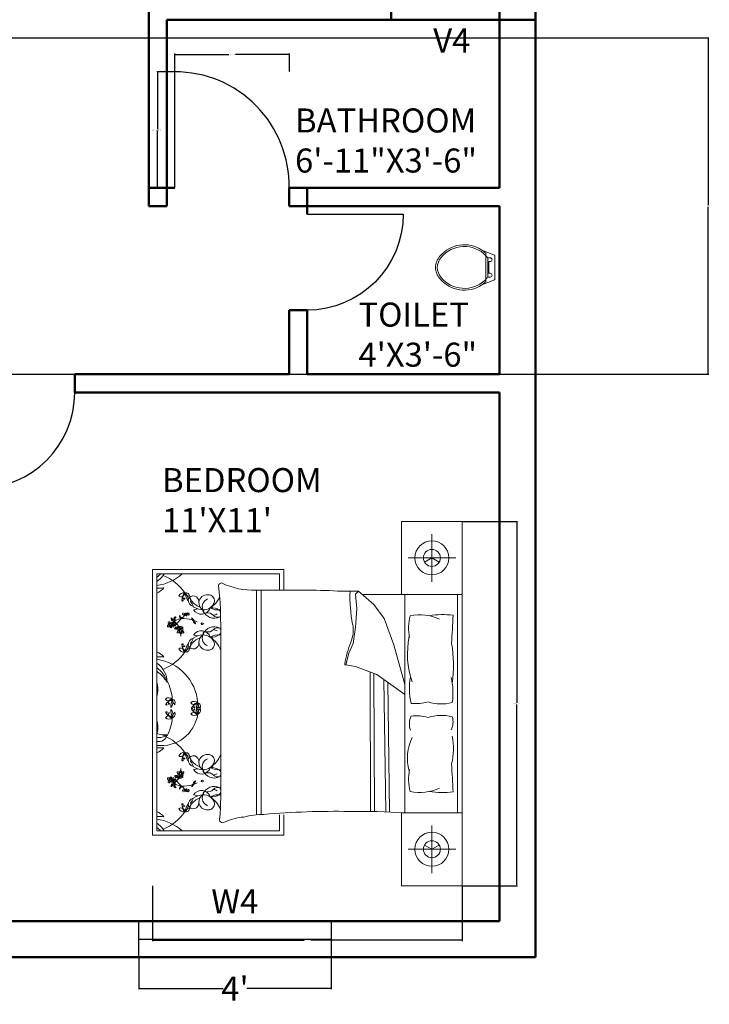
# Model space of a CAD drawing. Units: inches. Extents: x -173 to 545, y -746 to 104.
# Tile 19 of 32: x 373 to 545, y -709 to -463. Entities that reach past the tile are written whole.
import ezdxf

# ---------------------------------------------------------------- set-up
doc = ezdxf.new("R2010")
doc.units = ezdxf.units.IN
doc.header["$MEASUREMENT"] = 0
for name, color, linetype, lineweight in [('A-ANNO-DIMS', 2, 'Continuous', 18), ('A-ANNO-TEXT', 7, 'Continuous', 18), ('A-AREA-IDEN', 7, 'Continuous', 18), ('A-DOOR', 4, 'Continuous', 25), ('A-FLOR-FIXT', 8, 'Continuous', 18), ('A-FURN', 8, 'Continuous', 18), ('A-GLAZ', 3, 'Continuous', 25), ('A-WALL', 7, 'Continuous', 50)]:
    doc.layers.add(name, color=color, linetype=linetype, lineweight=lineweight)
doc.styles.get("Standard").update_dxf_attribs({"font": 'arial.ttf'})
doc.dimstyles.get("Standard").update_dxf_attribs({"dimtxt": 0.18, "dimasz": 0.18, "dimexe": 0.18, "dimexo": 0.0625, "dimgap": 0.09, "dimtad": 0, "dimtih": 1, "dimtoh": 1, "dimdec": 0, "dimzin": 0, "dimdsep": 46, "dimlunit": 3, "dimtxsty": 'Standard', "dimcen": 0.09, "dimadec": 0, "dimazin": 0, "dimtfac": 1, "dimtdec": 0, "dimtofl": 0, "dimtmove": 0, "dimatfit": 3, "dimfxl": 1, "dimtolj": 1, "dimtzin": 0, "dimarcsym": 0})

# ---------------------------------------------------------------- blocks, each defined once
blk = doc.blocks.new('*D20')
at = {"layer": 'A-ANNO-DIMS', "color": 0, "lineweight": -2, "transparency": 16777216}
for p, q in [((402.8, -697.42), (402.8, -705.33)), ((450.8, -697.42), (450.8, -705.33)), ((402.98, -705.15), (423.83, -705.15)), ((450.62, -705.15), (429.77, -705.15))]:
    blk.add_line(p, q, dxfattribs=at)
at = {"layer": 'A-ANNO-DIMS', "color": 0, "transparency": 16777216}
for points in [[(402.98, -705.12), (402.98, -705.18), (402.8, -705.15)], [(450.62, -705.12), (450.62, -705.18), (450.8, -705.15)]]:
    blk.add_solid(points, dxfattribs=at)
at = {"layer": 'Defpoints', "color": 0, "transparency": 16777216}
for p in [(402.8, -697.36), (450.8, -697.36), (450.8, -705.15)]:
    blk.add_point(p, dxfattribs=at)
at = {"layer": 'A-ANNO-DIMS', "color": 0, "transparency": 16777216, "insert": (426.8, -705.15), "char_height": 6, "attachment_point": 5}
blk.add_mtext("\\A1;4'", dxfattribs=at)
blk = doc.blocks.new('BED-SUITE-LARGE')
for p, q in [((77.28, 90.87), (77.28, 0)), ((69.71, 75.85), (69.71, 87.72)), ((63.77, 81.79), (75.65, 81.79)), ((0, 78.88), (32.74, 78.88)), ((0, 12.63), (0, 78.88)), ((32.74, 78.88), (32.74, 73.74)), ((1.05, 77.83), (1.05, 13.68)), ((31.68, 77.83), (1.05, 77.83)), ((31.68, 73.74), (31.68, 77.83)), ((25.93, 17.68), (25.93, 73.75)), ((27.07, 17.76), (27.07, 73.75)), ((50.66, 72.78), (51.39, 73.51)), ((51.02, 69.09), (50.66, 72.78)), ((51.39, 73.51), (55.25, 70.2)), ((77.28, 72.7), (52.34, 72.7)), ((62.92, 72.7), (62.92, 18.17)), ((76.12, 18.17), (76.12, 72.7)), ((10.27, 68.87), (11.29, 69.07)), ((50.66, 64.49), (51.02, 69.09)), ((55.25, 70.2), (57.83, 66.7)), ((57.83, 66.7), (60.22, 60.08)), ((50.1, 60.44), (50.66, 64.49)), ((10.27, 62.52), (11.29, 62.32)), ((17.01, 26.99), (17.01, 63.88)), ((49, 58.05), (50.1, 60.44)), ((60.22, 60.08), (62.92, 50.17)), ((48.26, 55.11), (49, 58.05)), ((50.66, 54.74), (48.26, 55.11)), ((55.99, 52.71), (50.66, 54.74)), ((54.42, 18.5), (54.28, 53.36)), ((55.35, 18.5), (55.22, 53.01)), ((62.92, 47.73), (55.99, 52.71)), ((58.21, 18.45), (57.75, 51.45)), ((59.15, 18.42), (58.69, 50.77)), ((10.27, 28.99), (11.29, 29.19)), ((10.27, 22.64), (11.29, 22.44)), ((31.68, 13.68), (31.68, 17.69)), ((32.74, 17.67), (32.74, 12.63)), ((69.71, 15.02), (69.71, 3.15)), ((32.74, 12.63), (0, 12.63)), ((1.05, 13.68), (31.68, 13.68)), ((63.77, 9.09), (75.65, 9.09))]:
    blk.add_line(p, q)
for points in [[(62.14, 72.7), (62.14, 90.87), (77.28, 90.87)], [(69.71, 81.79), (67.87, 80.73)], [(69.71, 81.79), (71.55, 80.73)], [(77.28, 18.17), (62.14, 18.17), (62.14, 0), (77.28, 0)], [(69.71, 9.09), (67.87, 10.15)], [(69.71, 9.09), (71.55, 10.15)]]:
    blk.add_lwpolyline(points)
for points in [[(43.07, 73.7, 0.001242), (25.83, 73.75, -0.127202), (17.23, 75.57)], [(75.02, 67.48, 0.074897), (69.08, 67.37, -0.472817)], [(68.75, 45.86, 0.14099), (74.8, 45.68, 0.235245)], [(68.75, 41.98, -0.14099), (74.8, 42.16, -0.235245)], [(75.02, 23.39, -0.074897), (69.08, 23.5, 0.472817)], [(27.78, 17.79, 0.056112), (22.78, 17.13, 0.095341), (17.97, 15.85)]]:
    blk.add_lwpolyline(points, format="xyb")
for centre, radius in [((69.71, 81.79), 4.24), ((69.71, 81.79), 2.12), ((4.53, 65.13), 0.231), ((6.97, 63.62), 0.231), ((6.97, 27.89), 0.231), ((4.53, 26.37), 0.231), ((69.71, 9.09), 4.24), ((69.71, 9.09), 2.12)]:
    blk.add_circle(centre, radius)
for centre, radius, start, end in [((-3.21, 82.79), 7.21, 306.3036, 316.4814), ((-2.13, 80.71), 5.78, 303.4617, 330.1116), ((-0.55, 86.66), 11.87, 277.745, 311.8856), ((-1.72, 66.36), 11.87, 34.3865, 68.5908), ((-0.8, 77.47), 4.82, 292.5547, 318.9546), ((1.8, 90.69), 16.42, 267.4081, 273.6519), ((17.29, 74.73), 0.838, 93.98, 207.3412), ((-77.59, 64.97), 94.6, 359.3433, 5.6887), ((7.79, 71.77), 1.32, 77.7115, 159.0387), ((7.08, 73.09), 0.991, 238.4633, 358.2869), ((10.33, 71.08), 3, 138.8402, 177.9352), ((7.56, 71.2), 0.0716, 11.4834, 127.9409), ((8.52, 72.2), 0.971, 117.6827, 223.7762), ((7.92, 71.62), 0.128, 223.7762, 159.7183), ((8.31, 72.1), 0.984, 2.9516, 103.728), ((16.18, 74.86), 8.3, 192.5173, 207.1824), ((6.98, 71.54), 1.88, 345.4653, 54.2343), ((9.8, 74.12), 2.03, 211.3827, 255.2969), ((10.19, 70.95), 1.36, 350.264, 160.8688), ((10.6, 71.28), 1.7, 175.969, 254.3045), ((8.71, 71.23), 0.836, 333.9755, 53.2681), ((13.19, 73.65), 4.29, 211.2614, 251.7045), ((13.69, 70.45), 2.17, 84.9449, 172.8857), ((14.51, 69.6), 2.11, 111.5819, 201.4221), ((13.91, 71.08), 1.53, 354.4856, 91.0538), ((10.61, 75.09), 6.88, 303.6671, 333.2997), ((49.13, 156.83), 83.35, 265.8294, 271.553), ((83.57, 71.96), 34.3, 177.4519, 191.3392), ((7.48, 71.19), 0.147, 177.9352, 11.4834), ((8.34, 69.44), 1.81, 6.1662, 51.5825), ((12.85, 73.69), 4.88, 236.2883, 266.5076), ((12.22, 70), 2.26, 209.9085, 343.1337), ((14.17, 70.83), 2.64, 182.3591, 234.0401), ((12.78, 71.55), 2.73, 265.2933, 346.921), ((14.7, 65.87), 3.5, 122.7011, 126.3445), ((16.34, 72.56), 3.76, 238.8218, 279.1554), ((14.7, 65.87), 3.5, 55.785, 94.7304), ((4.87, 66.63), 0.258, 124.3538, 214.3923), ((5.25, 66.59), 0.602, 190.3057, 287.1958), ((5.42, 66.8), 0.7, 176.9701, 248.2913), ((10.42, 70.49), 6.76, 212.6784, 216.3746), ((5.19, 66.64), 0.268, 216.3746, 291.7548), ((5.83, 66.45), 0.602, 122.8155, 187.3992), ((5.36, 66.2), 0.202, 289.3605, 111.7548), ((6.09, 66.37), 0.7, 109.4799, 177.6828), ((5.72, 66.82), 0.258, 56.8636, 146.9021), ((5.85, 66.53), 0.268, 148.8844, 224.2646), ((11.41, 63.17), 6.76, 145.1882, 148.8844), ((7.56, 62.88), 3.77, 94.756, 119.2041), ((15.59, 57.45), 12.42, 132.2412, 142.1744), ((9.32, 67.33), 2.56, 178.3264, 187.1302), ((6.55, 66.98), 0.477, 11.3256, 64.4621), ((8.17, 67.67), 1.44, 190.2588, 210.656), ((7.21, 67.08), 0.436, 188.3432, 274.2869), ((7.59, 67.32), 0.762, 210.656, 242.6341), ((8.17, 67.98), 1.46, 218.2101, 226.3071), ((7.09, 66.75), 0.185, 325.7657, 67.4417), ((1.34, 72.94), 8.63, 313.1541, 322.0459), ((7.74, 59.14), 7.53, 73.5842, 93.8277), ((7.69, 67.76), 0.178, 142.4737, 265.053), ((7.92, 67.79), 0.382, 127.7621, 169.0403), ((7.72, 68.11), 0.538, 265.053, 338.3618), ((8.43, 67.38), 0.703, 113.4276, 137.6104), ((8.35, 68.11), 0.231, 183.2768, 356.7232), ((8.52, 67.69), 0.379, 139.7889, 227.6792), ((8.4, 67.56), 0.199, 227.6792, 350.3487), ((7.63, 67.69), 0.758, 353.0852, 15.7171), ((8.12, 67.6), 0.478, 350.3487, 43.6538), ((9.01, 68.1), 0.557, 198.7263, 262.5032), ((8.57, 67.84), 0.221, 1.1081, 91.8675), ((8.71, 67.79), 0.386, 11.5637, 52.6358), ((8.98, 67.72), 0.179, 255.2356, 54.9248), ((12.38, 66.79), 2.56, 178.3264, 187.1302), ((9.61, 66.44), 0.477, 11.3256, 64.4621), ((11.23, 67.12), 1.44, 190.2588, 210.656), ((10.27, 66.54), 0.436, 188.3432, 274.2869), ((10.65, 66.78), 0.762, 210.656, 242.6341), ((11.23, 67.43), 1.46, 218.2101, 226.3071), ((10.15, 66.21), 0.185, 325.7657, 67.4417), ((13.17, 68.57), 0.564, 167.3041, 285.1471), ((15.36, 69.65), 2.9, 199.2822, 299.1751), ((13.81, 66.22), 1.86, 41.5653, 105.1471), ((14.83, 70.08), 2.61, 277.436, 299.9149), ((16.22, 68.36), 1.36, 221.5653, 293.8354), ((16, 67.9), 1.09, 30.0293, 52.325), ((16, 67.9), 1.09, 314.4517, 333.558), ((76.08, 64.24), 12.18, 165.1039, 191.0369), ((66.7, 55.9), 11.71, 65.1316, 101.7583), ((939.83, 17.39), 866.26, 176.68521, 177.14978), ((3.87, 64.78), 0.178, 142.4737, 265.053), ((4.11, 64.82), 0.382, 61.2196, 169.0403), ((3.9, 65.14), 0.538, 265.053, 338.3618), ((4.36, 65.61), 0.457, 157.4086, 261.4386), ((4.1, 65.62), 0.229, 58.0499, 135.6268), ((4.61, 64.41), 0.703, 113.4276, 137.6104), ((4.34, 65.48), 0.153, 172.906, 277.132), ((3.83, 65.2), 0.73, 14.7558, 58.0499), ((4.7, 64.72), 0.379, 139.7889, 227.6792), ((4.58, 64.58), 0.199, 227.6792, 350.3487), ((4.86, 65.39), 0.316, 36.1046, 181.4281), ((3.81, 64.72), 0.758, 353.0852, 15.7171), ((4.31, 64.63), 0.478, 350.3487, 43.6538), ((4.67, 65.64), 0.319, 270.0645, 331.1507), ((4.94, 65.56), 0.364, 221.8413, 265.7877), ((5.19, 65.12), 0.557, 198.7263, 262.5032), ((4.75, 64.86), 0.221, 1.1081, 91.8675), ((4.94, 65.42), 0.227, 263.7526, 41.7054), ((4.89, 64.81), 0.386, 11.5637, 86.365), ((7.56, 62.88), 3.77, 124.0033, 132.4917), ((5.17, 64.75), 0.179, 255.2356, 54.9248), ((3.67, 62.41), 4.03, 63.7819, 68.2913), ((5.83, 65.51), 0.641, 128.3208, 208.8162), ((5.94, 65.56), 0.766, 207.7043, 254.3516), ((5.51, 66.2), 0.202, 221.8703, 44.2646), ((6.43, 65.62), 1.05, 157.2305, 229.0635), ((6.07, 65.96), 0.621, 174.4544, 220.6188), ((5.44, 65.12), 1.05, 270.278, 342.111), ((6.15, 63.8), 0.746, 98.7227, 159.3375), ((5.77, 64.76), 0.766, 244.9899, 291.6373), ((2.54, 62.5), 4.53, 30.544, 49.818), ((5.04, 65.07), 0.746, 340.0041, 40.6188), ((5.94, 65.15), 0.621, 278.7227, 324.8872), ((5.83, 64.65), 0.641, 290.5253, 358.5375), ((6.8, 64.09), 0.457, 157.4086, 261.4386), ((6.54, 64.11), 0.229, 58.0499, 135.6268), ((7.08, 64.83), 0.641, 182.8499, 266.1226), ((6.83, 65.28), 0.621, 231.7607, 277.9252), ((7.32, 65.39), 1.05, 214.5369, 286.3699), ((6.78, 63.96), 0.153, 172.906, 277.132), ((6.27, 63.68), 0.73, 14.7558, 58.0499), ((2.54, 62.5), 4.53, 23.0501, 23.8477), ((7.02, 63.93), 0.746, 37.3105, 97.9252), ((7.3, 63.88), 0.316, 36.1046, 181.4281), ((7.11, 64.95), 0.766, 265.0106, 311.658), ((7.11, 64.12), 0.319, 270.0645, 331.1507), ((7.38, 63.91), 0.227, 263.7526, 41.7054), ((10.67, 65.87), 0.436, 147.5332, 233.4768), ((11.06, 66.09), 0.762, 179.1859, 211.164), ((10.32, 65.92), 0.185, 354.3784, 96.0543), ((7.74, 59.14), 7.53, 63.0032, 69.8941), ((11.64, 66.44), 1.44, 211.164, 231.5612), ((11.89, 67.61), 2.56, 234.6898, 243.4936), ((11.91, 66.29), 1.46, 195.5129, 203.6099), ((10.27, 65.34), 0.477, 357.3579, 50.4944), ((12.32, 65.43), 0.175, 12.7051, 190.4384), ((12.43, 65.45), 0.285, 190.4384, 10.4136), ((15.36, 61.74), 2.9, 60.8249, 160.7178), ((13.81, 65.17), 1.86, 254.8529, 318.4347), ((14.83, 61.31), 2.61, 60.0851, 82.564), ((16.22, 63.03), 1.36, 66.1646, 138.4347), ((16, 63.49), 1.09, 23.229, 45.5483), ((42.69, 63.76), 7.4, 336.2616, 11.3392), ((6.31, 63.27), 0.178, 142.4737, 265.053), ((6.54, 63.31), 0.382, 61.2196, 169.0403), ((6.34, 63.63), 0.538, 265.053, 338.3618), ((7.05, 62.89), 0.703, 113.4276, 137.6104), ((7.14, 63.2), 0.379, 139.7889, 227.6792), ((7.02, 63.07), 0.199, 227.6792, 350.3487), ((6.25, 63.21), 0.758, 353.0852, 15.7171), ((2.54, 62.5), 4.53, 357.1071, 4.7585), ((6.75, 63.12), 0.478, 350.3487, 43.6538), ((7.38, 64.05), 0.364, 221.8413, 265.7877), ((7.63, 63.61), 0.557, 198.7263, 262.5032), ((7.19, 63.35), 0.221, 1.1081, 91.8675), ((7.33, 63.3), 0.386, 11.5637, 86.365), ((7.61, 63.23), 0.179, 255.2356, 54.9248), ((10.6, 60.11), 1.7, 105.6955, 184.031), ((8.34, 61.95), 1.81, 308.4175, 353.8338), ((13.19, 57.74), 4.29, 108.2955, 148.7386), ((12.85, 57.7), 4.88, 93.4924, 123.7117), ((12.22, 61.39), 2.26, 16.8663, 150.0915), ((14.17, 60.56), 2.64, 125.9599, 177.6409), ((14.51, 61.79), 2.11, 158.5779, 248.4181), ((12.78, 59.84), 2.73, 13.079, 94.7067), ((13.17, 62.82), 0.564, 74.8529, 192.6959), ((14.7, 65.52), 3.5, 233.6555, 237.2989), ((16.34, 58.83), 3.76, 79.7133, 121.1782), ((14.7, 65.52), 3.5, 265.2696, 304.215), ((10.61, 56.3), 6.88, 21.4941, 56.3329), ((16, 63.49), 1.09, 307.675, 336.7144), ((84.74, 57.83), 21.12, 168.0397, 199.2615), ((7.08, 58.3), 0.991, 1.7131, 121.5367), ((7.79, 59.62), 1.32, 200.9613, 282.2885), ((7.48, 60.2), 0.147, 348.5166, 182.0648), ((10.33, 60.31), 3, 182.0648, 221.1598), ((7.56, 60.19), 0.0716, 232.0591, 348.5166), ((8.52, 59.19), 0.971, 136.2238, 242.3173), ((7.97, 59.76), 0.0774, 200.2667, 136.2271), ((6.98, 59.85), 1.88, 305.7657, 14.5347), ((16.18, 56.53), 8.3, 152.8176, 167.4827), ((8.31, 59.29), 0.984, 256.272, 357.0484), ((9.8, 57.27), 2.03, 104.7031, 148.6173), ((10.19, 60.44), 1.36, 199.1312, 9.736), ((8.71, 60.16), 0.836, 306.7319, 26.0245), ((13.69, 60.94), 2.17, 187.1143, 275.0551), ((13.91, 60.31), 1.53, 268.9462, 5.5144), ((82.6, 48.8), 35.24, 160.1194, 169.3383), ((42.13, 55.03), 32.96, 352.2196, 9.497), ((-0.8, 53.92), 4.82, 41.0454, 67.4453), ((1.8, 40.7), 16.42, 86.3481, 92.5919), ((-1.72, 65.03), 11.87, 291.4092, 325.6135), ((-0.55, 44.73), 11.87, 4.4623, 82.255), ((-2.13, 50.68), 5.78, 1.272, 56.5383), ((-3.21, 48.6), 7.21, 17.8504, 53.6964), ((48.19, 55.31), 0.219, 178.8623, 289.7536), ((-5.24, 44.82), 10.72, 34.0123, 54.053), ((80.12, 49.28), 16.03, 169.8617, 193.6238), ((58.79, 48.07), 16.19, 351.5249, 13.96), ((-5.19, 48.96), 6.53, 343.5431, 17.0202), ((-6.9, 45.64), 11.87, 4.4623, 27.4146), ((-8.55, 46.37), 9.65, 4.3787, 5.6357), ((-15.16, 41.29), 17.24, 19.7217, 19.9028), ((4.04, 45.59), 1.32, 47.7873, 129.1145), ((4.09, 47.08), 0.991, 208.5391, 328.3627), ((3.48, 45.23), 0.147, 148.011, 341.5592), ((5.9, 43.72), 3, 108.9159, 148.011), ((3.55, 45.21), 0.0716, 341.5592, 98.0167), ((4.89, 45.59), 0.971, 87.7585, 193.852), ((4.07, 45.39), 0.128, 193.852, 129.9245), ((12.85, 44.08), 8.3, 162.593, 177.2582), ((3.22, 45.79), 1.88, 315.5411, 24.3101), ((6.96, 46.61), 2.03, 181.4585, 225.3727), ((4.65, 45.62), 0.984, 333.0274, 73.8037), ((10.4, 44.68), 1.32, 47.7873, 129.1145), ((10.44, 46.17), 0.991, 208.5391, 328.3627), ((9.84, 44.33), 0.147, 148.011, 341.5592), ((9.84, 44.15), 0.147, 18.4408, 211.989), ((12.26, 42.81), 3, 108.9159, 148.011), ((9.91, 44.3), 0.0716, 341.5592, 98.0167), ((11.25, 44.68), 0.971, 87.7585, 193.852), ((10.43, 44.48), 0.128, 193.852, 129.9245), ((9.58, 44.88), 1.88, 315.5411, 24.3101), ((19.21, 43.17), 8.3, 162.593, 177.2582), ((9.58, 43.6), 1.88, 335.6899, 44.4589), ((19.21, 45.31), 8.3, 182.7418, 197.407), ((11.01, 44.71), 0.984, 333.0274, 73.8037), ((13.31, 45.7), 2.03, 181.4585, 225.3727), ((65.71, 56.57), 11.13, 264.0129, 285.8293), ((2.19, 44.13), 9.18, 262.8636, 351.8197), ((4.09, 41.4), 0.991, 31.6373, 151.4609), ((4.04, 42.89), 1.32, 230.8855, 312.2127), ((3.48, 43.24), 0.147, 18.4408, 211.989), ((5.9, 44.75), 3, 211.989, 251.0841), ((3.55, 43.27), 0.0716, 261.9833, 18.4408), ((-6.9, 42.84), 11.87, 332.5854, 355.5377), ((4.89, 42.89), 0.971, 166.148, 272.2415), ((4.12, 43.1), 0.0774, 230.1909, 166.0209), ((12.85, 44.4), 8.3, 182.7418, 197.407), ((3.22, 42.69), 1.88, 335.6899, 44.4589), ((6.96, 41.86), 2.03, 134.6273, 178.5415), ((4.65, 42.86), 0.984, 286.1963, 26.9726), ((10.44, 42.3), 0.991, 31.6373, 151.4609), ((10.4, 43.8), 1.32, 230.8855, 312.2127), ((12.26, 45.66), 3, 211.989, 251.0841), ((9.91, 44.18), 0.0716, 261.9833, 18.4408), ((11.25, 43.79), 0.971, 166.148, 272.2415), ((10.48, 44.01), 0.0774, 230.1909, 166.0209), ((11.01, 43.77), 0.984, 286.1963, 26.9726), ((13.31, 42.77), 2.03, 134.6273, 178.5415), ((68.92, 40.31), 4.82, 155.0183, 198.5407), ((65.71, 31.27), 11.13, 74.1707, 95.9871), ((70.49, 40.92), 4.5, 333.3437, 16.1026), ((-5.19, 39.52), 6.53, 342.9798, 16.4569), ((-8.55, 42.11), 9.65, 354.3643, 355.6213), ((-15.16, 47.19), 17.24, 340.0972, 340.2783), ((3.03, 42.94), 5.31, 248.117, 276.6195), ((1.55, 38.07), 2.13, 256.3898, 349.0739), ((1.85, 39.67), 2.69, 252.8609, 311.9049), ((-1.72, 26.47), 11.87, 34.3865, 68.5908), ((75.18, 31.89), 11.57, 153.8761, 196.1746), ((59.12, 34.18), 15.97, 346.3427, 11.1841), ((1.8, 50.8), 16.42, 267.4081, 273.6519), ((-0.8, 37.59), 4.82, 292.5547, 318.9546), ((7.79, 31.89), 1.32, 77.7115, 159.0387), ((7.08, 33.21), 0.991, 238.4633, 358.2869), ((10.33, 31.2), 3, 138.8402, 177.9352), ((8.52, 32.32), 0.971, 117.6827, 223.7762), ((8.31, 32.22), 0.984, 2.9516, 103.728), ((9.8, 34.23), 2.03, 211.3827, 255.2969), ((6.98, 31.65), 1.88, 345.4653, 54.2343), ((16.18, 34.98), 8.3, 192.5173, 207.1824), ((10.19, 31.07), 1.36, 350.264, 160.8688), ((8.71, 31.35), 0.836, 333.9755, 53.2681), ((13.69, 30.57), 2.17, 84.9449, 172.8857), ((13.91, 31.2), 1.53, 354.4856, 91.0538), ((10.61, 35.2), 6.88, 303.6671, 338.5059), ((7.48, 31.3), 0.147, 177.9352, 11.4834), ((7.56, 31.32), 0.0716, 11.4834, 127.9409), ((7.92, 31.73), 0.128, 223.7762, 159.7183), ((10.6, 31.39), 1.7, 175.969, 254.3045), ((8.34, 29.56), 1.81, 6.1662, 51.5825), ((13.19, 33.77), 4.29, 211.2614, 251.7045), ((12.85, 33.81), 4.88, 236.2883, 266.5076), ((14.17, 30.94), 2.64, 182.3591, 234.0401), ((14.51, 29.71), 2.11, 111.5819, 201.4221), ((12.78, 31.67), 2.73, 265.2933, 346.921), ((14.7, 25.98), 3.5, 55.785, 94.7304), ((939.83, 73.48), 866.26, 182.85022, 183.31479), ((4.7, 26.79), 0.379, 132.3208, 220.2111), ((4.58, 26.92), 0.199, 9.6513, 132.3208), ((5.77, 26.75), 0.766, 68.3627, 115.0101), ((5.44, 26.39), 1.05, 17.889, 89.722), ((6.15, 27.71), 0.746, 200.6625, 261.2773), ((5.83, 26.86), 0.641, 1.4625, 69.4747), ((6.31, 28.24), 0.178, 94.947, 217.5263), ((6.54, 28.2), 0.382, 190.9597, 298.7804), ((6.34, 27.88), 0.538, 21.6382, 94.947), ((6.8, 27.42), 0.457, 98.5614, 202.5914), ((6.54, 27.4), 0.229, 224.3732, 301.9501), ((7.08, 26.68), 0.641, 93.8774, 177.1501), ((7.32, 26.11), 1.05, 73.6301, 145.4631), ((7.05, 28.61), 0.703, 222.3896, 246.5724), ((6.78, 27.54), 0.153, 82.868, 187.094), ((6.27, 27.82), 0.73, 301.9501, 345.2442), ((2.54, 29.01), 4.53, 336.1523, 336.9499), ((7.14, 28.3), 0.379, 132.3208, 220.2111), ((7.02, 28.44), 0.199, 9.6513, 132.3208), ((7.02, 27.58), 0.746, 262.0748, 322.6895), ((6.25, 28.3), 0.758, 344.2829, 6.9148), ((7.3, 27.63), 0.316, 178.5719, 323.8954), ((7.11, 26.55), 0.766, 48.342, 94.9894), ((2.54, 29.01), 4.53, 355.2415, 2.8929), ((6.75, 28.39), 0.478, 316.3462, 9.6513), ((7.63, 27.9), 0.557, 97.4968, 161.2737), ((7.38, 27.46), 0.364, 94.2123, 138.1587), ((7.11, 27.38), 0.319, 28.8493, 89.9355), ((7.19, 28.16), 0.221, 268.1325, 358.8919), ((7.33, 28.21), 0.386, 273.635, 348.4363), ((7.38, 27.6), 0.227, 318.2946, 96.2474), ((7.61, 28.28), 0.179, 305.0752, 104.7644), ((12.22, 30.11), 2.26, 209.9085, 343.1337), ((13.17, 28.68), 0.564, 167.3041, 285.1471), ((14.7, 25.98), 3.5, 122.7011, 126.3445), ((15.36, 29.76), 2.9, 199.2822, 299.1751), ((13.81, 26.34), 1.86, 41.5653, 105.1471), ((16.34, 32.68), 3.76, 238.8218, 280.2867), ((14.83, 30.2), 2.61, 277.436, 299.9149), ((16.22, 28.48), 1.36, 221.5653, 293.8354), ((16, 28.02), 1.09, 23.2856, 52.325), ((16, 28.02), 1.09, 314.4517, 336.7144), ((76.08, 26.64), 12.18, 168.9631, 194.8961), ((3.87, 26.72), 0.178, 94.947, 217.5263), ((4.11, 26.69), 0.382, 190.9597, 298.7804), ((3.9, 26.36), 0.538, 21.6382, 94.947), ((4.36, 25.9), 0.457, 98.5614, 202.5914), ((4.1, 25.89), 0.229, 224.3732, 301.9501), ((4.61, 27.1), 0.703, 222.3896, 246.5724), ((4.34, 26.03), 0.153, 82.868, 187.094), ((3.83, 26.31), 0.73, 301.9501, 345.2442), ((3.81, 26.79), 0.758, 344.2829, 6.9148), ((4.86, 26.12), 0.316, 178.5719, 323.8954), ((4.87, 24.88), 0.258, 145.6077, 235.6462), ((4.31, 26.88), 0.478, 316.3462, 9.6513), ((5.25, 24.92), 0.602, 72.8042, 169.6943), ((5.19, 26.38), 0.557, 97.4968, 161.2737), ((4.94, 25.94), 0.364, 94.2123, 138.1587), ((4.67, 25.87), 0.319, 28.8493, 89.9355), ((5.42, 24.7), 0.7, 111.7087, 183.0299), ((10.42, 21.02), 6.76, 143.6254, 147.3216), ((4.75, 26.64), 0.221, 268.1325, 358.8919), ((4.89, 26.69), 0.386, 273.635, 348.4363), ((4.94, 26.08), 0.227, 318.2946, 96.2474), ((5.19, 24.87), 0.268, 68.2452, 143.6254), ((7.56, 28.62), 3.77, 227.5083, 235.9967), ((5.17, 26.76), 0.179, 305.0752, 104.7644), ((3.67, 29.1), 4.03, 291.7087, 296.2181), ((5.83, 26), 0.641, 151.1838, 231.6792), ((5.83, 25.05), 0.602, 172.6008, 237.1845), ((5.94, 25.95), 0.766, 105.6484, 152.2957), ((5.36, 25.3), 0.202, 248.2452, 70.6395), ((5.51, 25.3), 0.202, 315.7354, 138.1297), ((6.43, 25.89), 1.05, 130.9365, 202.7695), ((6.09, 25.13), 0.7, 182.3172, 250.5201), ((6.07, 25.54), 0.621, 139.3812, 185.5456), ((2.54, 29.01), 4.53, 310.182, 329.456), ((5.85, 24.98), 0.268, 135.7354, 211.1156), ((5.04, 26.43), 0.746, 319.3812, 19.9959), ((11.41, 28.33), 6.76, 211.1156, 214.8118), ((7.56, 28.62), 3.77, 240.7959, 265.244), ((15.59, 34.05), 12.42, 217.8256, 227.7588), ((5.94, 26.36), 0.621, 35.1128, 81.2773), ((6.83, 26.23), 0.621, 82.0748, 128.2393), ((8.17, 23.84), 1.44, 149.344, 169.7412), ((7.21, 24.43), 0.436, 85.7131, 171.6568), ((7.59, 24.19), 0.762, 117.3659, 149.344), ((8.17, 23.53), 1.46, 133.6929, 141.7899), ((7.09, 24.76), 0.185, 292.5583, 34.2343), ((7.74, 32.37), 7.53, 266.1723, 286.4158), ((1.34, 18.57), 8.63, 37.9541, 46.8459), ((11.23, 24.38), 1.44, 149.344, 169.7412), ((12.38, 24.71), 2.56, 172.8698, 181.6736), ((9.61, 25.07), 0.477, 295.5379, 348.6744), ((10.27, 24.97), 0.436, 85.7131, 171.6568), ((10.65, 24.73), 0.762, 117.3659, 149.344), ((11.23, 24.07), 1.46, 133.6929, 141.7899), ((10.15, 25.3), 0.185, 292.5583, 34.2343), ((10.67, 25.64), 0.436, 126.5232, 212.4668), ((11.06, 25.41), 0.762, 148.836, 180.8141), ((10.32, 25.59), 0.185, 263.9457, 5.6216), ((7.74, 32.37), 7.53, 290.1059, 296.9968), ((11.64, 25.06), 1.44, 128.4388, 148.836), ((11.89, 23.9), 2.56, 116.5064, 125.3102), ((11.91, 25.21), 1.46, 156.3901, 164.4871), ((10.27, 26.17), 0.477, 309.5056, 2.6421), ((12.32, 26.07), 0.175, 169.5616, 347.2949), ((12.43, 26.05), 0.285, 349.5864, 169.5616), ((15.36, 21.86), 2.9, 60.8249, 160.7178), ((-71.37, 24.21), 88.43, 355.2402, 1.8035), ((5.72, 24.69), 0.258, 213.0979, 303.1364), ((9.32, 24.17), 2.56, 172.8698, 181.6736), ((6.55, 24.53), 0.477, 295.5379, 348.6744), ((7.69, 23.75), 0.178, 94.947, 217.5263), ((7.92, 23.72), 0.382, 190.9597, 232.2379), ((7.72, 23.39), 0.538, 21.6382, 94.947), ((8.43, 24.13), 0.703, 222.3896, 246.5724), ((8.35, 23.4), 0.231, 3.2768, 176.7232), ((8.52, 23.82), 0.379, 132.3208, 220.2111), ((8.4, 23.95), 0.199, 9.6513, 132.3208), ((7.63, 23.81), 0.758, 344.2829, 6.9148), ((8.12, 23.9), 0.478, 316.3462, 9.6513), ((9.01, 23.41), 0.557, 97.4968, 161.2737), ((8.57, 23.67), 0.221, 268.1325, 358.8919), ((8.98, 23.79), 0.179, 305.0752, 104.7644), ((8.71, 23.72), 0.386, 307.3642, 348.4363), ((12.85, 17.81), 4.88, 93.4924, 123.7117), ((12.22, 21.51), 2.26, 16.8663, 150.0915), ((14.17, 20.68), 2.64, 125.9599, 177.6409), ((14.51, 21.91), 2.11, 158.5779, 248.4181), ((12.78, 19.96), 2.73, 13.079, 94.7067), ((13.17, 22.94), 0.564, 74.8529, 192.6959), ((14.7, 25.64), 3.5, 233.6555, 237.2989), ((13.81, 25.28), 1.86, 254.8529, 318.4347), ((16.34, 18.94), 3.76, 79.249, 121.1782), ((14.7, 25.64), 3.5, 265.2696, 304.215), ((10.61, 16.42), 6.88, 23.6453, 56.3329), ((14.83, 21.42), 2.61, 60.0851, 82.564), ((16.22, 23.14), 1.36, 66.1646, 138.4347), ((16, 23.61), 1.09, 307.675, 342.5814), ((16, 23.61), 1.09, 16.6343, 45.5483), ((66.7, 34.97), 11.71, 258.2417, 294.8684), ((7.48, 20.32), 0.147, 348.5166, 182.0648), ((10.33, 20.42), 3, 182.0648, 221.1598), ((7.56, 20.3), 0.0716, 232.0591, 348.5166), ((8.52, 19.31), 0.971, 136.2238, 242.3173), ((7.97, 19.88), 0.0774, 200.2667, 136.2271), ((16.18, 16.65), 8.3, 152.8176, 167.4827), ((6.98, 19.97), 1.88, 305.7657, 14.5347), ((10.6, 20.23), 1.7, 105.6955, 184.031), ((10.19, 20.56), 1.36, 199.1312, 9.736), ((8.71, 20.28), 0.836, 306.7319, 26.0245), ((8.34, 22.06), 1.81, 308.4175, 353.8338), ((13.19, 17.85), 4.29, 108.2955, 148.7386), ((13.69, 21.06), 2.17, 187.1143, 275.0551), ((13.91, 20.43), 1.53, 268.9462, 5.5144), ((-0.8, 14.04), 4.82, 41.0454, 67.4453), ((1.8, 0.82), 16.42, 86.3481, 92.5919), ((-1.72, 25.15), 11.87, 291.4092, 325.6135), ((7.08, 18.42), 0.991, 1.7131, 121.5367), ((7.79, 19.73), 1.32, 200.9613, 282.2885), ((9.8, 17.39), 2.03, 104.7031, 148.6173), ((8.31, 19.4), 0.984, 256.272, 357.0484), ((45.88, -194.44), 213, 89.1145, 94.8735), ((51.82, -144.73), 163.28, 86.1, 90.9282), ((-0.55, 4.85), 11.87, 48.1144, 82.255), ((-2.13, 10.8), 5.78, 29.8884, 56.5383), ((17.51, 16.54), 0.828, 156.5219, 303.8264), ((-3.21, 8.72), 7.21, 43.5186, 53.6964)]:
    blk.add_arc(centre, radius, start, end)
blk = doc.blocks.new('WC-STANDARD')
for p, q in [((12.59, 8.59), (12.59, 9.21)), ((12.59, 8.59), (12.59, 5.67)), ((12.59, 2.75), (12.59, 5.67)), ((12.59, 2.13), (12.59, 2.75))]:
    blk.add_line(p, q)
for points in [[(11.57, 10.01, 0.383919), (1.07, 8.46, 0.163732), (0, 5.67, 0.359733)], [(12.59, 8.59, 0.448546), (1.41, 8.18, 0.162618), (0.44, 5.67, 0.470877)], [(12.59, 9.21, 0.040937), (11.57, 10.01, 0.163732)], [(14.84, 5.67), (14.84, 8.5, 0.31031), (14.6, 8.85), (11.57, 10.01, 0.209071)], [(13.04, 8.08, 0.022712), (12.59, 8.59, 0.162618)], [(13.04, 5.67), (13.04, 8.08, 0.476108)], [(13.04, 8.08), (13.66, 8.08, -1), (13.66, 7.13), (13.34, 7.13)], [(11.57, 1.32, -0.383919), (1.07, 2.88, -0.163732), (0, 5.67, -0.359733)], [(12.29, 2.45, -0.431639), (1.41, 3.16, -0.162618), (0.44, 5.67, -0.470877)], [(14.84, 5.67), (14.84, 2.84, -0.31031), (14.6, 2.49), (11.57, 1.32, -0.209071)], [(13.04, 5.67), (13.04, 3.26, -0.022712)], [(12.59, 2.75, -0.014165), (12.29, 2.45, -0.162618)], [(13.04, 3.26, -0.022712), (12.59, 2.75, -0.162618)], [(13.04, 3.26), (13.66, 3.26, 1), (13.66, 4.21), (13.34, 4.21)], [(12.59, 2.13, -0.040937), (11.57, 1.32, -0.163732)]]:
    blk.add_lwpolyline(points, format="xyb")
for points in [[(13.34, 7.13), (13.04, 7.13)], [(13.34, 7.13), (13.34, 4.21)], [(13.34, 4.21), (13.04, 4.21)]]:
    blk.add_lwpolyline(points)
blk = doc.blocks.new('WINDOW-48')
for p, q in [((0, 9), (48, 9)), ((0, 0), (0, 9)), ((48, 9), (48, 0)), ((0, 4.5), (48, 4.5)), ((48, 0), (0, 0))]:
    blk.add_line(p, q)
blk = doc.blocks.new('DOOR-24')
blk.add_line((24, 0), (24, 24))
blk.add_arc((24, 0), 24, 90, 180)
blk = doc.blocks.new('DOOR-BATH-29')
for p, q in [((28.5, 29), (28.5, 5)), ((28.5, 5), (28.5, 0))]:
    blk.add_line(p, q)
blk.add_arc((28.5, 28.5), 28.5, 179.0036, 270)
blk = doc.blocks.new('*D56')
at = {"layer": 'A-ANNO-DIMS', "color": 0, "lineweight": -2, "transparency": 16777216}
for p, q in [((411.74, -476.36), (407.27, -476.36)), ((407.45, -476.54), (407.45, -490.68)), ((407.45, -505.18), (407.45, -491.05)), ((411.74, -505.36), (407.27, -505.36))]:
    blk.add_line(p, q, dxfattribs=at)
at = {"layer": 'A-ANNO-DIMS', "color": 0, "transparency": 16777216}
for points in [[(407.42, -476.54), (407.48, -476.54), (407.45, -476.36)], [(407.42, -505.18), (407.48, -505.18), (407.45, -505.36)]]:
    blk.add_solid(points, dxfattribs=at)
at = {"layer": 'Defpoints', "color": 0, "transparency": 16777216}
for p in [(411.8, -476.36), (407.45, -505.36), (411.8, -505.36)]:
    blk.add_point(p, dxfattribs=at)
at = {"layer": 'A-ANNO-DIMS', "color": 0, "transparency": 16777216, "insert": (407.45, -490.86), "char_height": 0.18, "attachment_point": 5}
blk.add_mtext('\\A1;BATH DOOR 2\'-5" TYP.', dxfattribs=at)
blk = doc.blocks.new('*D57')
at = {"layer": 'A-ANNO-DIMS', "color": 0, "lineweight": -2, "transparency": 16777216}
for p, q in [((411.8, -476.3), (411.8, -471.83)), ((411.98, -472.01), (425.27, -472.01)), ((440.25, -472.01), (426.97, -472.01)), ((440.43, -476.3), (440.43, -471.83))]:
    blk.add_line(p, q, dxfattribs=at)
at = {"layer": 'A-ANNO-DIMS', "color": 0, "transparency": 16777216}
for points in [[(411.98, -471.98), (411.98, -472.04), (411.8, -472.01)], [(440.25, -471.98), (440.25, -472.04), (440.43, -472.01)]]:
    blk.add_solid(points, dxfattribs=at)
at = {"layer": 'Defpoints', "color": 0, "transparency": 16777216}
for p in [(411.8, -472.01), (411.8, -476.36), (440.43, -476.36)]:
    blk.add_point(p, dxfattribs=at)
at = {"layer": 'A-ANNO-DIMS', "color": 0, "transparency": 16777216, "insert": (426.12, -472.01), "char_height": 0.18, "attachment_point": 5}
blk.add_mtext('\\A1;2\'-4 1/2" TYP.', dxfattribs=at)
blk = doc.blocks.new('*D60')
at = {"layer": 'A-ANNO-DIMS', "color": 0, "lineweight": -2, "transparency": 16777216}
for p, q in [((483.58, -588.61), (497.33, -588.61)), ((497.15, -588.79), (497.15, -633.86)), ((497.15, -679.3), (497.15, -634.23)), ((483.58, -679.48), (497.33, -679.48))]:
    blk.add_line(p, q, dxfattribs=at)
at = {"layer": 'A-ANNO-DIMS', "color": 0, "transparency": 16777216}
for points in [[(497.12, -588.79), (497.18, -588.79), (497.15, -588.61)], [(497.12, -679.3), (497.18, -679.3), (497.15, -679.48)]]:
    blk.add_solid(points, dxfattribs=at)
at = {"layer": 'Defpoints', "color": 0, "transparency": 16777216}
for p in [(483.51, -588.61), (497.15, -588.61), (483.51, -679.48)]:
    blk.add_point(p, dxfattribs=at)
at = {"layer": 'A-ANNO-DIMS', "color": 0, "transparency": 16777216, "insert": (497.15, -634.04), "char_height": 0.18, "attachment_point": 5}
blk.add_mtext('\\A1;BED SET 7\'-7" TYP.', dxfattribs=at)
blk = doc.blocks.new('*D61')
at = {"layer": 'A-ANNO-DIMS', "color": 0, "lineweight": -2, "transparency": 16777216}
for p, q in [((406.23, -679.54), (406.23, -693.29)), ((483.51, -679.54), (483.51, -693.29)), ((406.41, -693.11), (444.03, -693.11)), ((483.33, -693.11), (445.72, -693.11))]:
    blk.add_line(p, q, dxfattribs=at)
at = {"layer": 'A-ANNO-DIMS', "color": 0, "transparency": 16777216}
for points in [[(406.41, -693.08), (406.41, -693.14), (406.23, -693.11)], [(483.33, -693.08), (483.33, -693.14), (483.51, -693.11)]]:
    blk.add_solid(points, dxfattribs=at)
at = {"layer": 'Defpoints', "color": 0, "transparency": 16777216}
for p in [(406.23, -679.48), (483.51, -679.48), (483.51, -693.11)]:
    blk.add_point(p, dxfattribs=at)
at = {"layer": 'A-ANNO-DIMS', "color": 0, "transparency": 16777216, "insert": (444.87, -693.11), "char_height": 0.18, "attachment_point": 5}
blk.add_mtext('\\A1;6\'-5 1/2" TYP.', dxfattribs=at)
blk = doc.blocks.new('*D82')
at = {"layer": 'A-ANNO-DIMS', "color": 0, "lineweight": -2, "transparency": 16777216}
for p, q in [((219.86, -467.86), (545.08, -467.86)), ((544.9, -468.04), (544.9, -509.68)), ((544.9, -551.68), (544.9, -510.04)), ((219.86, -551.86), (545.08, -551.86))]:
    blk.add_line(p, q, dxfattribs=at)
at = {"layer": 'A-ANNO-DIMS', "color": 0, "transparency": 16777216}
for points in [[(544.87, -468.04), (544.93, -468.04), (544.9, -467.86)], [(544.87, -551.68), (544.93, -551.68), (544.9, -551.86)]]:
    blk.add_solid(points, dxfattribs=at)
at = {"layer": 'Defpoints', "color": 0, "transparency": 16777216}
for p in [(219.8, -467.86), (219.8, -551.86), (544.9, -551.86)]:
    blk.add_point(p, dxfattribs=at)
at = {"layer": 'A-ANNO-DIMS', "color": 0, "transparency": 16777216, "insert": (544.9, -509.86), "char_height": 0.18, "attachment_point": 5}
blk.add_mtext('\\A1;7\'-0"', dxfattribs=at)

msp = doc.modelspace()

# ---------------------------------------------------------------- linework, layer by layer
at = {"layer": 'A-WALL'}
for p, q in [((501.8, 7.64), (501.8, -697.36)), ((465.8, -370.86), (465.8, -463.36)), ((405.3, -458.86), (405.3, -505.36)), ((492.8, -458.86), (492.8, -505.36)), ((409.8, -463.36), (409.8, -505.36)), ((409.8, -463.36), (501.8, -463.36)), ((411.8, -505.36), (405.3, -505.36)), ((405.3, -509.86), (405.3, -505.36)), ((409.8, -505.36), (409.8, -509.86)), ((440.3, -505.36), (492.8, -505.36)), ((440.3, -505.36), (440.3, -509.86)), ((444.8, -505.36), (444.8, -511.86)), ((409.8, -509.86), (405.3, -509.86)), ((440.3, -509.86), (492.8, -509.86)), ((492.8, -509.86), (492.8, -551.86)), ((444.8, -535.86), (440.3, -535.86)), ((440.3, -535.86), (440.3, -551.86)), ((444.8, -535.86), (444.8, -551.86)), ((386.8, -551.86), (440.3, -551.86)), ((386.8, -556.36), (386.8, -551.86)), ((444.8, -551.86), (492.8, -551.86)), ((386.8, -556.36), (492.8, -556.36)), ((492.8, -556.36), (492.8, -688.36)), ((360.8, -688.36), (492.8, -688.36)), ((24.3, -697.36), (501.8, -697.36))]:
    msp.add_line(p, q, dxfattribs=at)

# ---------------------------------------------------------------- block references
at = {"layer": 'A-DOOR', "rotation": 180}
for name, p in [('DOOR-BATH-29', (440.3, -476.36)), ('DOOR-24', (386.8, -556.36))]:
    msp.add_blockref(name, p, dxfattribs=at)
at = {"layer": 'A-DOOR', "extrusion": (0, 0, -1), "zscale": -1, "rotation": 89.99999999999989}
msp.add_blockref('DOOR-24', (-444.8, -535.86), dxfattribs=at)
at = {"layer": 'A-FLOR-FIXT'}
msp.add_blockref('WC-STANDARD', (476.84, -530.86), dxfattribs=at)
at = {"layer": 'A-FURN'}
msp.add_blockref('BED-SUITE-LARGE', (406.23, -679.48), dxfattribs=at)
at = {"layer": 'A-GLAZ'}
msp.add_blockref('WINDOW-48', (402.8, -697.36), dxfattribs=at)

# ---------------------------------------------------------------- texts
at = {"layer": 'A-ANNO-TEXT', "char_height": 6, "attachment_point": 1}
for s, insert in [('V4', (476.28, -465.56)), ('W4', (420.89, -680.41))]:
    msp.add_mtext(s, dxfattribs=dict(at, insert=insert))
at = {"layer": 'A-AREA-IDEN', "char_height": 6, "attachment_point": 1}
for s, insert in [('BATHROOM\\P6\'-11"X3\'-6"', (441.8, -485.51)), ("BEDROOM\\P11'X11'", (408.61, -575.26))]:
    msp.add_mtext(s, dxfattribs=dict(at, insert=insert))
at = {"layer": 'A-AREA-IDEN', "insert": (457.63, -533.96), "char_height": 6, "attachment_point": 1}
msp.add_mtext_dynamic_manual_height_columns('TOILET\\P4\'X3\'-6"', width=0.2125, gutter_width=1, heights=[0], dxfattribs=at)

# ---------------------------------------------------------------- dimensions: what is measured, and where the dimension line sits
at = {"layer": 'A-ANNO-DIMS'}
dim = msp.add_linear_dim(base=(544.9, -551.86), p1=(219.8, -467.86), p2=(219.8, -551.86), angle=90, dimstyle='Standard', override={"dimdec": 1, "dimlfac": 1, "dimrnd": 0, "dimzin": 1, "dimdsep": 46, "dimlunit": 4, "dimfrac": 2}, dxfattribs=at)
dim.commit()
dim.dimension.update_dxf_attribs({"geometry": '*D82', "text_midpoint": (544.9, -509.86)})
for base, p1, p2, angle, text, picture, middle in [((411.8, -472.01), (440.43, -476.36), (411.8, -476.36), 180, '<> TYP.', '*D57', (426.12, -472.01)), ((407.45, -505.36), (411.8, -476.36), (411.8, -505.36), 270, 'BATH DOOR <> TYP.', '*D56', (407.45, -490.86)), ((497.15, -588.61), (483.51, -679.48), (483.51, -588.61), 90, 'BED SET <> TYP.', '*D60', (497.15, -634.04))]:
    dim = msp.add_linear_dim(base=base, p1=p1, p2=p2, angle=angle, text=text, dimstyle='Standard', override={"dimdec": 1, "dimlfac": 1, "dimrnd": 0, "dimzin": 1, "dimdsep": 46, "dimlunit": 4, "dimfrac": 2}, dxfattribs=at)
    dim.commit()
    dim.dimension.update_dxf_attribs({"geometry": picture, "text_midpoint": middle})
dim = msp.add_linear_dim(base=(483.51, -693.11), p1=(406.23, -679.48), p2=(483.51, -679.48), text='<> TYP.', dimstyle='Standard', override={"dimdec": 1, "dimlfac": 1, "dimrnd": 0, "dimzin": 1, "dimdsep": 46, "dimlunit": 4, "dimfrac": 2}, dxfattribs=at)
dim.commit()
dim.dimension.update_dxf_attribs({"geometry": '*D61', "text_midpoint": (444.87, -693.11)})
dim = msp.add_linear_dim(base=(450.8, -705.15), p1=(402.8, -697.36), p2=(450.8, -697.36), dimstyle='Standard', override={"dimtxt": 6, "dimclrd": 0, "dimclre": 0, "dimclrt": 0}, dxfattribs=at)
dim.commit()
dim.dimension.update_dxf_attribs({"geometry": '*D20', "text_midpoint": (426.8, -705.15)})

doc.saveas('drawing.dxf')
